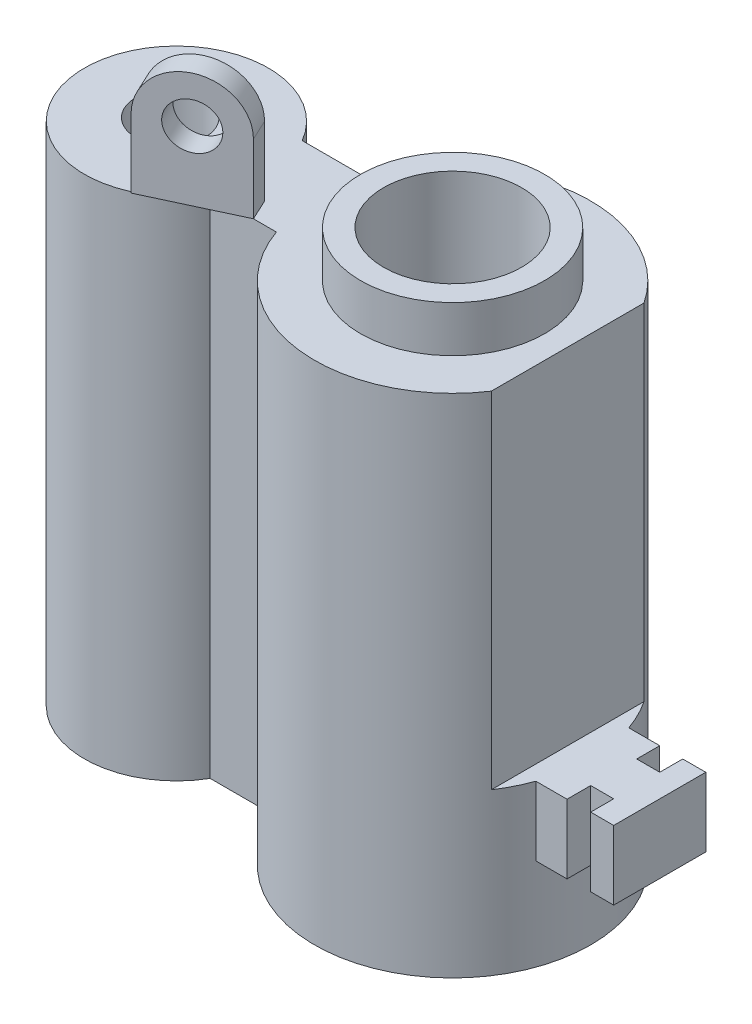
ISO-10303-21;
HEADER;
FILE_DESCRIPTION(('STEP AP214'),'2;1');
FILE_NAME('part.step','',(''),(''),'','','');
FILE_SCHEMA(('AUTOMOTIVE_DESIGN { 1 0 10303 214 1 1 1 1 }'));
ENDSEC;
DATA;
#1=APPLICATION_CONTEXT('core data for automotive mechanical design processes');
#2=APPLICATION_PROTOCOL_DEFINITION('international standard','automotive_design',2000,#1);
#3=PRODUCT_CONTEXT('',#1,'mechanical');
#4=PRODUCT('Part','Part','',(#3));
#5=PRODUCT_RELATED_PRODUCT_CATEGORY('part','',(#4));
#6=PRODUCT_DEFINITION_FORMATION('','',#4);
#7=PRODUCT_DEFINITION_CONTEXT('part definition',#1,'design');
#8=PRODUCT_DEFINITION('design','',#6,#7);
#9=PRODUCT_DEFINITION_SHAPE('','',#8);
#10=(LENGTH_UNIT() NAMED_UNIT(*) SI_UNIT(.MILLI.,.METRE.));
#11=(NAMED_UNIT(*) PLANE_ANGLE_UNIT() SI_UNIT($,.RADIAN.));
#12=(NAMED_UNIT(*) SI_UNIT($,.STERADIAN.) SOLID_ANGLE_UNIT());
#13=UNCERTAINTY_MEASURE_WITH_UNIT(LENGTH_MEASURE(1.E-05),#10,'distance_accuracy_value','');
#14=(GEOMETRIC_REPRESENTATION_CONTEXT(3) GLOBAL_UNCERTAINTY_ASSIGNED_CONTEXT((#13)) GLOBAL_UNIT_ASSIGNED_CONTEXT((#10,
#11,#12)) REPRESENTATION_CONTEXT('',''));
#15=CARTESIAN_POINT('',(0.,0.,0.));
#16=DIRECTION('',(0.,0.,1.));
#17=DIRECTION('',(1.,0.,0.));
#18=AXIS2_PLACEMENT_3D('',#15,#16,#17);
#19=CARTESIAN_POINT('',(0.,22.,0.));
#20=DIRECTION('',(0.,-1.,0.));
#21=DIRECTION('',(0.,0.,-1.));
#22=AXIS2_PLACEMENT_3D('',#19,#20,#21);
#23=CYLINDRICAL_SURFACE('',#22,6.);
#24=DIRECTION('',(0.,-1.,0.));
#25=VECTOR('',#24,1.);
#26=CARTESIAN_POINT('',(5.,27.,-3.3166247903554));
#27=LINE('',#26,#25);
#28=CARTESIAN_POINT('',(5.,22.,-3.3166247903554));
#29=VERTEX_POINT('',#28);
#30=CARTESIAN_POINT('',(5.,7.,-3.3166247903554));
#31=VERTEX_POINT('',#30);
#32=EDGE_CURVE('E215',#29,#31,#27,.T.);
#33=ORIENTED_EDGE('',*,*,#32,.T.);
#34=CARTESIAN_POINT('',(0.,7.,0.));
#35=DIRECTION('',(0.,1.,0.));
#36=DIRECTION('',(0.,0.,1.));
#37=AXIS2_PLACEMENT_3D('',#34,#35,#36);
#38=CIRCLE('',#37,6.);
#39=CARTESIAN_POINT('',(5.65685424949238,7.,-2.));
#40=VERTEX_POINT('',#39);
#41=EDGE_CURVE('E199',#40,#31,#38,.T.);
#42=ORIENTED_EDGE('',*,*,#41,.F.);
#43=DIRECTION('',(0.,1.,0.));
#44=VECTOR('',#43,1.);
#45=CARTESIAN_POINT('',(5.65685424949238,4.,-2.));
#46=LINE('',#45,#44);
#47=CARTESIAN_POINT('',(5.65685424949238,4.,-2.));
#48=VERTEX_POINT('',#47);
#49=EDGE_CURVE('E288',#48,#40,#46,.T.);
#50=ORIENTED_EDGE('',*,*,#49,.F.);
#51=CARTESIAN_POINT('',(0.,4.,0.));
#52=DIRECTION('',(0.,1.,0.));
#53=DIRECTION('',(0.,0.,1.));
#54=AXIS2_PLACEMENT_3D('',#51,#52,#53);
#55=CIRCLE('',#54,6.);
#56=CARTESIAN_POINT('',(5.64698166944062,4.,2.02770757877006));
#57=VERTEX_POINT('',#56);
#58=EDGE_CURVE('E46',#57,#48,#55,.T.);
#59=ORIENTED_EDGE('',*,*,#58,.F.);
#60=DIRECTION('',(0.,1.,0.));
#61=VECTOR('',#60,1.);
#62=CARTESIAN_POINT('',(5.64698166944062,4.,2.02770757877006));
#63=LINE('',#62,#61);
#64=CARTESIAN_POINT('',(5.64698166944062,7.,2.02770757877006));
#65=VERTEX_POINT('',#64);
#66=EDGE_CURVE('E259',#57,#65,#63,.T.);
#67=ORIENTED_EDGE('',*,*,#66,.T.);
#68=CARTESIAN_POINT('',(5.,7.,3.31662479035539));
#69=VERTEX_POINT('',#68);
#70=EDGE_CURVE('E206',#69,#65,#38,.T.);
#71=ORIENTED_EDGE('',*,*,#70,.F.);
#72=DIRECTION('',(0.,-1.,0.));
#73=VECTOR('',#72,1.);
#74=CARTESIAN_POINT('',(5.,27.,3.31662479035539));
#75=LINE('',#74,#73);
#76=CARTESIAN_POINT('',(5.,22.,3.31662479035539));
#77=VERTEX_POINT('',#76);
#78=EDGE_CURVE('E211',#77,#69,#75,.T.);
#79=ORIENTED_EDGE('',*,*,#78,.F.);
#80=CARTESIAN_POINT('',(0.,22.,0.));
#81=DIRECTION('',(0.,1.,0.));
#82=DIRECTION('',(0.,0.,1.));
#83=AXIS2_PLACEMENT_3D('',#80,#81,#82);
#84=CIRCLE('',#83,6.);
#85=CARTESIAN_POINT('',(-5.65685424949238,22.,2.));
#86=VERTEX_POINT('',#85);
#87=EDGE_CURVE('E373',#86,#77,#84,.T.);
#88=ORIENTED_EDGE('',*,*,#87,.F.);
#89=DIRECTION('',(0.,-1.,0.));
#90=VECTOR('',#89,1.);
#91=CARTESIAN_POINT('',(-5.65685424949238,22.,2.));
#92=LINE('',#91,#90);
#93=CARTESIAN_POINT('',(-5.65685424949238,0.,2.));
#94=VERTEX_POINT('',#93);
#95=EDGE_CURVE('E383',#86,#94,#92,.T.);
#96=ORIENTED_EDGE('',*,*,#95,.T.);
#97=CARTESIAN_POINT('',(0.,0.,0.));
#98=DIRECTION('',(0.,1.,0.));
#99=DIRECTION('',(0.,0.,1.));
#100=AXIS2_PLACEMENT_3D('',#97,#98,#99);
#101=CIRCLE('',#100,6.);
#102=CARTESIAN_POINT('',(-5.65685424949238,0.,-2.));
#103=VERTEX_POINT('',#102);
#104=EDGE_CURVE('E375',#94,#103,#101,.T.);
#105=ORIENTED_EDGE('',*,*,#104,.T.);
#106=DIRECTION('',(0.,-1.,0.));
#107=VECTOR('',#106,1.);
#108=CARTESIAN_POINT('',(-5.65685424949238,22.,-2.));
#109=LINE('',#108,#107);
#110=CARTESIAN_POINT('',(-5.65685424949238,22.,-2.));
#111=VERTEX_POINT('',#110);
#112=EDGE_CURVE('E405',#111,#103,#109,.T.);
#113=ORIENTED_EDGE('',*,*,#112,.F.);
#114=EDGE_CURVE('E220',#29,#111,#84,.T.);
#115=ORIENTED_EDGE('',*,*,#114,.F.);
#116=EDGE_LOOP('',(#33,#42,#50,#59,#67,#71,#79,#88,#96,#105,#113,#115));
#117=FACE_BOUND('',#116,.T.);
#118=ADVANCED_FACE('F39',(#117),#23,.T.);
#119=CARTESIAN_POINT('',(0.,22.,0.));
#120=DIRECTION('',(0.,1.,0.));
#121=DIRECTION('',(0.,0.,1.));
#122=AXIS2_PLACEMENT_3D('',#119,#120,#121);
#123=PLANE('',#122);
#124=CARTESIAN_POINT('',(0.,22.,0.));
#125=DIRECTION('',(0.,1.,0.));
#126=DIRECTION('',(0.,0.,1.));
#127=AXIS2_PLACEMENT_3D('',#124,#125,#126);
#128=CIRCLE('',#127,4.);
#129=CARTESIAN_POINT('',(0.,22.,4.));
#130=VERTEX_POINT('',#129);
#131=EDGE_CURVE('E317',#130,#130,#128,.T.);
#132=ORIENTED_EDGE('',*,*,#131,.F.);
#133=EDGE_LOOP('',(#132));
#134=FACE_BOUND('',#133,.T.);
#135=CARTESIAN_POINT('',(-12.2679491924311,22.,0.));
#136=DIRECTION('',(0.,1.,0.));
#137=DIRECTION('',(0.,0.,1.));
#138=AXIS2_PLACEMENT_3D('',#135,#136,#137);
#139=CIRCLE('',#138,1.5);
#140=CARTESIAN_POINT('',(-12.2679491924311,22.,1.5));
#141=VERTEX_POINT('',#140);
#142=EDGE_CURVE('E333',#141,#141,#139,.T.);
#143=ORIENTED_EDGE('',*,*,#142,.F.);
#144=EDGE_LOOP('',(#143));
#145=FACE_BOUND('',#144,.T.);
#146=ORIENTED_EDGE('',*,*,#87,.T.);
#147=DIRECTION('',(0.,0.,-1.));
#148=VECTOR('',#147,1.);
#149=CARTESIAN_POINT('',(5.,22.,0.));
#150=LINE('',#149,#148);
#151=EDGE_CURVE('E11',#77,#29,#150,.T.);
#152=ORIENTED_EDGE('',*,*,#151,.T.);
#153=ORIENTED_EDGE('',*,*,#114,.T.);
#154=DIRECTION('',(-1.,0.,0.));
#155=VECTOR('',#154,1.);
#156=CARTESIAN_POINT('',(-8.53589838486226,22.,-2.));
#157=LINE('',#156,#155);
#158=CARTESIAN_POINT('',(-8.53589838486226,22.,-2.));
#159=VERTEX_POINT('',#158);
#160=EDGE_CURVE('E376',#111,#159,#157,.T.);
#161=ORIENTED_EDGE('',*,*,#160,.T.);
#162=CARTESIAN_POINT('',(-12.,22.,0.));
#163=DIRECTION('',(0.,1.,0.));
#164=DIRECTION('',(0.,0.,1.));
#165=AXIS2_PLACEMENT_3D('',#162,#163,#164);
#166=CIRCLE('',#165,3.99999999999999);
#167=CARTESIAN_POINT('',(-10.3095269530372,22.,3.6252311481466));
#168=VERTEX_POINT('',#167);
#169=EDGE_CURVE('E378',#159,#168,#166,.T.);
#170=ORIENTED_EDGE('',*,*,#169,.T.);
#171=DIRECTION('',(0.422618261740698,0.,0.906307787036651));
#172=VECTOR('',#171,1.);
#173=CARTESIAN_POINT('',(-10.2791041559867,22.,3.69047304696279));
#174=LINE('',#173,#172);
#175=CARTESIAN_POINT('',(-10.7017224177274,22.,2.78416525992614));
#176=VERTEX_POINT('',#175);
#177=EDGE_CURVE('E52',#176,#168,#174,.T.);
#178=ORIENTED_EDGE('',*,*,#177,.F.);
#179=DIRECTION('',(-0.906307787036651,0.,0.422618261740697));
#180=VECTOR('',#179,1.);
#181=CARTESIAN_POINT('',(-10.7017224177274,22.,2.78416525992614));
#182=LINE('',#181,#180);
#183=CARTESIAN_POINT('',(-7.07649126958075,22.,1.09369221296335));
#184=VERTEX_POINT('',#183);
#185=EDGE_CURVE('E353',#184,#176,#182,.T.);
#186=ORIENTED_EDGE('',*,*,#185,.F.);
#187=DIRECTION('',(-0.422618261740697,0.,-0.906307787036651));
#188=VECTOR('',#187,1.);
#189=CARTESIAN_POINT('',(-7.07649126958075,22.,1.09369221296335));
#190=LINE('',#189,#188);
#191=CARTESIAN_POINT('',(-6.65387300784006,22.,2.));
#192=VERTEX_POINT('',#191);
#193=EDGE_CURVE('E56',#192,#184,#190,.T.);
#194=ORIENTED_EDGE('',*,*,#193,.F.);
#195=DIRECTION('',(1.,0.,0.));
#196=VECTOR('',#195,1.);
#197=CARTESIAN_POINT('',(-8.53589838486226,22.,2.));
#198=LINE('',#197,#196);
#199=EDGE_CURVE('E382',#192,#86,#198,.T.);
#200=ORIENTED_EDGE('',*,*,#199,.T.);
#201=EDGE_LOOP('',(#146,#152,#153,#161,#170,#178,#186,#194,#200));
#202=FACE_BOUND('',#201,.T.);
#203=ADVANCED_FACE('F452',(#134,#145,#202),#123,.T.);
#204=CARTESIAN_POINT('',(-8.53589838486226,22.,-2.));
#205=DIRECTION('',(0.,0.,1.));
#206=DIRECTION('',(1.,0.,0.));
#207=AXIS2_PLACEMENT_3D('',#204,#205,#206);
#208=PLANE('',#207);
#209=DIRECTION('',(-1.,0.,0.));
#210=VECTOR('',#209,1.);
#211=CARTESIAN_POINT('',(-8.53589838486226,0.,-2.));
#212=LINE('',#211,#210);
#213=CARTESIAN_POINT('',(-8.53589838486226,0.,-2.));
#214=VERTEX_POINT('',#213);
#215=EDGE_CURVE('E389',#103,#214,#212,.T.);
#216=ORIENTED_EDGE('',*,*,#215,.T.);
#217=DIRECTION('',(0.,-1.,0.));
#218=VECTOR('',#217,1.);
#219=CARTESIAN_POINT('',(-8.53589838486226,22.,-2.));
#220=LINE('',#219,#218);
#221=EDGE_CURVE('E399',#159,#214,#220,.T.);
#222=ORIENTED_EDGE('',*,*,#221,.F.);
#223=ORIENTED_EDGE('',*,*,#160,.F.);
#224=ORIENTED_EDGE('',*,*,#112,.T.);
#225=EDGE_LOOP('',(#216,#222,#223,#224));
#226=FACE_BOUND('',#225,.T.);
#227=ADVANCED_FACE('F464',(#226),#208,.F.);
#228=CARTESIAN_POINT('',(-12.,22.,0.));
#229=DIRECTION('',(0.,-1.,0.));
#230=DIRECTION('',(0.,0.,-1.));
#231=AXIS2_PLACEMENT_3D('',#228,#229,#230);
#232=CYLINDRICAL_SURFACE('',#231,3.99999999999999);
#233=CARTESIAN_POINT('',(-12.,0.,0.));
#234=DIRECTION('',(0.,1.,0.));
#235=DIRECTION('',(0.,0.,1.));
#236=AXIS2_PLACEMENT_3D('',#233,#234,#235);
#237=CIRCLE('',#236,3.99999999999999);
#238=CARTESIAN_POINT('',(-8.53589838486226,0.,2.));
#239=VERTEX_POINT('',#238);
#240=EDGE_CURVE('E388',#214,#239,#237,.T.);
#241=ORIENTED_EDGE('',*,*,#240,.T.);
#242=DIRECTION('',(0.,-1.,0.));
#243=VECTOR('',#242,1.);
#244=CARTESIAN_POINT('',(-8.53589838486226,22.,2.));
#245=LINE('',#244,#243);
#246=CARTESIAN_POINT('',(-8.53589838486226,22.,2.));
#247=VERTEX_POINT('',#246);
#248=EDGE_CURVE('E398',#247,#239,#245,.T.);
#249=ORIENTED_EDGE('',*,*,#248,.F.);
#250=EDGE_CURVE('E377',#168,#247,#166,.T.);
#251=ORIENTED_EDGE('',*,*,#250,.F.);
#252=ORIENTED_EDGE('',*,*,#169,.F.);
#253=ORIENTED_EDGE('',*,*,#221,.T.);
#254=EDGE_LOOP('',(#241,#249,#251,#252,#253));
#255=FACE_BOUND('',#254,.T.);
#256=ADVANCED_FACE('F509',(#255),#232,.T.);
#257=CARTESIAN_POINT('',(-8.53589838486226,22.,2.));
#258=DIRECTION('',(0.,0.,-1.));
#259=DIRECTION('',(-1.,0.,0.));
#260=AXIS2_PLACEMENT_3D('',#257,#258,#259);
#261=PLANE('',#260);
#262=DIRECTION('',(1.,0.,0.));
#263=VECTOR('',#262,1.);
#264=CARTESIAN_POINT('',(-8.53589838486226,0.,2.));
#265=LINE('',#264,#263);
#266=EDGE_CURVE('E391',#239,#94,#265,.T.);
#267=ORIENTED_EDGE('',*,*,#266,.T.);
#268=ORIENTED_EDGE('',*,*,#95,.F.);
#269=ORIENTED_EDGE('',*,*,#199,.F.);
#270=EDGE_CURVE('E385',#247,#192,#198,.T.);
#271=ORIENTED_EDGE('',*,*,#270,.F.);
#272=ORIENTED_EDGE('',*,*,#248,.T.);
#273=EDGE_LOOP('',(#267,#268,#269,#271,#272));
#274=FACE_BOUND('',#273,.T.);
#275=ADVANCED_FACE('F453',(#274),#261,.F.);
#276=CARTESIAN_POINT('',(0.,0.,0.));
#277=DIRECTION('',(0.,1.,0.));
#278=DIRECTION('',(0.,0.,1.));
#279=AXIS2_PLACEMENT_3D('',#276,#277,#278);
#280=PLANE('',#279);
#281=CARTESIAN_POINT('',(0.,0.,0.));
#282=DIRECTION('',(0.,1.,0.));
#283=DIRECTION('',(0.,0.,1.));
#284=AXIS2_PLACEMENT_3D('',#281,#282,#283);
#285=CIRCLE('',#284,3.);
#286=CARTESIAN_POINT('',(0.,0.,3.));
#287=VERTEX_POINT('',#286);
#288=EDGE_CURVE('E286',#287,#287,#285,.T.);
#289=ORIENTED_EDGE('',*,*,#288,.T.);
#290=EDGE_LOOP('',(#289));
#291=FACE_BOUND('',#290,.T.);
#292=CARTESIAN_POINT('',(-12.2679491924311,0.,0.));
#293=DIRECTION('',(0.,1.,0.));
#294=DIRECTION('',(0.,0.,1.));
#295=AXIS2_PLACEMENT_3D('',#292,#293,#294);
#296=CIRCLE('',#295,1.5);
#297=CARTESIAN_POINT('',(-12.2679491924311,0.,1.5));
#298=VERTEX_POINT('',#297);
#299=EDGE_CURVE('E323',#298,#298,#296,.T.);
#300=ORIENTED_EDGE('',*,*,#299,.T.);
#301=EDGE_LOOP('',(#300));
#302=FACE_BOUND('',#301,.T.);
#303=ORIENTED_EDGE('',*,*,#104,.F.);
#304=ORIENTED_EDGE('',*,*,#266,.F.);
#305=ORIENTED_EDGE('',*,*,#240,.F.);
#306=ORIENTED_EDGE('',*,*,#215,.F.);
#307=EDGE_LOOP('',(#303,#304,#305,#306));
#308=FACE_BOUND('',#307,.T.);
#309=ADVANCED_FACE('F458',(#291,#302,#308),#280,.F.);
#310=CARTESIAN_POINT('',(-10.2791041559867,25.,3.69047304696279));
#311=DIRECTION('',(0.906307787036651,0.,-0.422618261740698));
#312=DIRECTION('',(-0.422618261740698,0.,-0.906307787036651));
#313=AXIS2_PLACEMENT_3D('',#310,#311,#312);
#314=PLANE('',#313);
#315=ORIENTED_EDGE('',*,*,#177,.T.);
#316=CARTESIAN_POINT('',(-10.2791041559867,22.,3.69047304696279));
#317=VERTEX_POINT('',#316);
#318=EDGE_CURVE('E341',#168,#317,#174,.T.);
#319=ORIENTED_EDGE('',*,*,#318,.T.);
#320=DIRECTION('',(0.,-1.,0.));
#321=VECTOR('',#320,1.);
#322=CARTESIAN_POINT('',(-10.2791041559867,25.,3.69047304696279));
#323=LINE('',#322,#321);
#324=CARTESIAN_POINT('',(-10.2791041559867,25.,3.69047304696279));
#325=VERTEX_POINT('',#324);
#326=EDGE_CURVE('E367',#325,#317,#323,.T.);
#327=ORIENTED_EDGE('',*,*,#326,.F.);
#328=DIRECTION('',(0.422618261740698,0.,0.906307787036651));
#329=VECTOR('',#328,1.);
#330=CARTESIAN_POINT('',(-10.2791041559867,25.,3.69047304696279));
#331=LINE('',#330,#329);
#332=CARTESIAN_POINT('',(-10.7017224177274,25.,2.78416525992614));
#333=VERTEX_POINT('',#332);
#334=EDGE_CURVE('E346',#333,#325,#331,.T.);
#335=ORIENTED_EDGE('',*,*,#334,.F.);
#336=DIRECTION('',(0.,-1.,0.));
#337=VECTOR('',#336,1.);
#338=CARTESIAN_POINT('',(-10.7017224177274,25.,2.78416525992614));
#339=LINE('',#338,#337);
#340=EDGE_CURVE('E354',#333,#176,#339,.T.);
#341=ORIENTED_EDGE('',*,*,#340,.T.);
#342=EDGE_LOOP('',(#315,#319,#327,#335,#341));
#343=FACE_BOUND('',#342,.T.);
#344=ADVANCED_FACE('F474',(#343),#314,.F.);
#345=CARTESIAN_POINT('',(-6.65387300784006,25.,2.));
#346=DIRECTION('',(-0.422618261740697,0.,-0.906307787036651));
#347=DIRECTION('',(-0.906307787036651,0.,0.422618261740698));
#348=AXIS2_PLACEMENT_3D('',#345,#346,#347);
#349=PLANE('',#348);
#350=CARTESIAN_POINT('',(-8.46648858191335,25.,2.8452365234814));
#351=DIRECTION('',(0.422618261740698,0.,0.906307787036651));
#352=DIRECTION('',(0.906307787036651,0.,-0.422618261740698));
#353=AXIS2_PLACEMENT_3D('',#350,#351,#352);
#354=CIRCLE('',#353,1.);
#355=CARTESIAN_POINT('',(-7.5601807948767,25.,2.4226182617407));
#356=VERTEX_POINT('',#355);
#357=EDGE_CURVE('E334',#356,#356,#354,.T.);
#358=ORIENTED_EDGE('',*,*,#357,.F.);
#359=EDGE_LOOP('',(#358));
#360=FACE_BOUND('',#359,.T.);
#361=DIRECTION('',(0.906307787036651,0.,-0.422618261740697));
#362=VECTOR('',#361,1.);
#363=CARTESIAN_POINT('',(-6.65387300784006,22.,2.));
#364=LINE('',#363,#362);
#365=EDGE_CURVE('E358',#317,#192,#364,.T.);
#366=ORIENTED_EDGE('',*,*,#365,.T.);
#367=DIRECTION('',(0.,-1.,0.));
#368=VECTOR('',#367,1.);
#369=CARTESIAN_POINT('',(-6.65387300784006,25.,2.));
#370=LINE('',#369,#368);
#371=CARTESIAN_POINT('',(-6.65387300784006,25.,2.));
#372=VERTEX_POINT('',#371);
#373=EDGE_CURVE('E366',#372,#192,#370,.T.);
#374=ORIENTED_EDGE('',*,*,#373,.F.);
#375=CARTESIAN_POINT('',(-8.46648858191336,25.,2.8452365234814));
#376=DIRECTION('',(0.422618261740698,0.,0.906307787036651));
#377=DIRECTION('',(0.906307787036651,0.,-0.422618261740698));
#378=AXIS2_PLACEMENT_3D('',#375,#376,#377);
#379=CIRCLE('',#378,2.);
#380=EDGE_CURVE('E336',#372,#325,#379,.T.);
#381=ORIENTED_EDGE('',*,*,#380,.T.);
#382=ORIENTED_EDGE('',*,*,#326,.T.);
#383=EDGE_LOOP('',(#366,#374,#381,#382));
#384=FACE_BOUND('',#383,.T.);
#385=ADVANCED_FACE('F481',(#360,#384),#349,.F.);
#386=CARTESIAN_POINT('',(-7.07649126958075,25.,1.09369221296335));
#387=DIRECTION('',(-0.906307787036651,0.,0.422618261740697));
#388=DIRECTION('',(0.422618261740697,0.,0.906307787036651));
#389=AXIS2_PLACEMENT_3D('',#386,#387,#388);
#390=PLANE('',#389);
#391=ORIENTED_EDGE('',*,*,#193,.T.);
#392=DIRECTION('',(0.,-1.,0.));
#393=VECTOR('',#392,1.);
#394=CARTESIAN_POINT('',(-7.07649126958075,25.,1.09369221296335));
#395=LINE('',#394,#393);
#396=CARTESIAN_POINT('',(-7.07649126958075,25.,1.09369221296335));
#397=VERTEX_POINT('',#396);
#398=EDGE_CURVE('E361',#397,#184,#395,.T.);
#399=ORIENTED_EDGE('',*,*,#398,.F.);
#400=DIRECTION('',(-0.422618261740697,0.,-0.906307787036651));
#401=VECTOR('',#400,1.);
#402=CARTESIAN_POINT('',(-7.07649126958075,25.,1.09369221296335));
#403=LINE('',#402,#401);
#404=EDGE_CURVE('E347',#372,#397,#403,.T.);
#405=ORIENTED_EDGE('',*,*,#404,.F.);
#406=ORIENTED_EDGE('',*,*,#373,.T.);
#407=EDGE_LOOP('',(#391,#399,#405,#406));
#408=FACE_BOUND('',#407,.T.);
#409=ADVANCED_FACE('F478',(#408),#390,.F.);
#410=CARTESIAN_POINT('',(-10.7017224177274,25.,2.78416525992614));
#411=DIRECTION('',(0.422618261740697,0.,0.906307787036651));
#412=DIRECTION('',(0.906307787036651,0.,-0.422618261740697));
#413=AXIS2_PLACEMENT_3D('',#410,#411,#412);
#414=PLANE('',#413);
#415=CARTESIAN_POINT('',(-8.88910684365405,25.,1.93892873644474));
#416=DIRECTION('',(0.422618261740698,0.,0.906307787036651));
#417=DIRECTION('',(0.906307787036651,0.,-0.422618261740698));
#418=AXIS2_PLACEMENT_3D('',#415,#416,#417);
#419=CIRCLE('',#418,1.);
#420=CARTESIAN_POINT('',(-7.9827990566174,25.,1.51631047470405));
#421=VERTEX_POINT('',#420);
#422=EDGE_CURVE('E332',#421,#421,#419,.T.);
#423=ORIENTED_EDGE('',*,*,#422,.T.);
#424=EDGE_LOOP('',(#423));
#425=FACE_BOUND('',#424,.T.);
#426=ORIENTED_EDGE('',*,*,#185,.T.);
#427=ORIENTED_EDGE('',*,*,#340,.F.);
#428=CARTESIAN_POINT('',(-8.88910684365406,25.,1.93892873644475));
#429=DIRECTION('',(0.422618261740698,0.,0.906307787036651));
#430=DIRECTION('',(0.906307787036651,0.,-0.422618261740698));
#431=AXIS2_PLACEMENT_3D('',#428,#429,#430);
#432=CIRCLE('',#431,2.);
#433=EDGE_CURVE('E342',#397,#333,#432,.T.);
#434=ORIENTED_EDGE('',*,*,#433,.F.);
#435=ORIENTED_EDGE('',*,*,#398,.T.);
#436=EDGE_LOOP('',(#426,#427,#434,#435));
#437=FACE_BOUND('',#436,.T.);
#438=ADVANCED_FACE('F476',(#425,#437),#414,.F.);
#439=CARTESIAN_POINT('',(0.,22.,0.));
#440=DIRECTION('',(0.,-1.,0.));
#441=DIRECTION('',(0.,0.,-1.));
#442=AXIS2_PLACEMENT_3D('',#439,#440,#441);
#443=PLANE('',#442);
#444=ORIENTED_EDGE('',*,*,#318,.F.);
#445=ORIENTED_EDGE('',*,*,#250,.T.);
#446=ORIENTED_EDGE('',*,*,#270,.T.);
#447=ORIENTED_EDGE('',*,*,#365,.F.);
#448=EDGE_LOOP('',(#444,#445,#446,#447));
#449=FACE_BOUND('',#448,.T.);
#450=ADVANCED_FACE('F472',(#449),#443,.T.);
#451=CARTESIAN_POINT('',(-8.88910684365406,25.,1.93892873644475));
#452=DIRECTION('',(0.422618261740698,0.,0.906307787036651));
#453=DIRECTION('',(0.906307787036651,0.,-0.422618261740698));
#454=AXIS2_PLACEMENT_3D('',#451,#452,#453);
#455=CYLINDRICAL_SURFACE('',#454,2.);
#456=ORIENTED_EDGE('',*,*,#380,.F.);
#457=ORIENTED_EDGE('',*,*,#404,.T.);
#458=ORIENTED_EDGE('',*,*,#433,.T.);
#459=ORIENTED_EDGE('',*,*,#334,.T.);
#460=EDGE_LOOP('',(#456,#457,#458,#459));
#461=FACE_BOUND('',#460,.T.);
#462=ADVANCED_FACE('F482',(#461),#455,.T.);
#463=CARTESIAN_POINT('',(-8.88910684365405,25.,1.93892873644474));
#464=DIRECTION('',(0.422618261740698,0.,0.906307787036651));
#465=DIRECTION('',(0.906307787036651,0.,-0.422618261740698));
#466=AXIS2_PLACEMENT_3D('',#463,#464,#465);
#467=CYLINDRICAL_SURFACE('',#466,1.);
#468=ORIENTED_EDGE('',*,*,#422,.F.);
#469=EDGE_LOOP('',(#468));
#470=FACE_BOUND('',#469,.T.);
#471=ORIENTED_EDGE('',*,*,#357,.T.);
#472=EDGE_LOOP('',(#471));
#473=FACE_BOUND('',#472,.T.);
#474=ADVANCED_FACE('F487',(#470,#473),#467,.F.);
#475=CARTESIAN_POINT('',(-12.2679491924311,22.,0.));
#476=DIRECTION('',(0.,1.,0.));
#477=DIRECTION('',(0.,0.,1.));
#478=AXIS2_PLACEMENT_3D('',#475,#476,#477);
#479=CYLINDRICAL_SURFACE('',#478,1.5);
#480=CARTESIAN_POINT('',(-12.2679491924311,16.,0.));
#481=DIRECTION('',(0.,1.,0.));
#482=DIRECTION('',(0.,0.,1.));
#483=AXIS2_PLACEMENT_3D('',#480,#481,#482);
#484=CIRCLE('',#483,1.5);
#485=CARTESIAN_POINT('',(-12.2679491924311,16.,1.5));
#486=VERTEX_POINT('',#485);
#487=EDGE_CURVE('E330',#486,#486,#484,.T.);
#488=ORIENTED_EDGE('',*,*,#487,.F.);
#489=EDGE_LOOP('',(#488));
#490=FACE_BOUND('',#489,.T.);
#491=ORIENTED_EDGE('',*,*,#142,.T.);
#492=EDGE_LOOP('',(#491));
#493=FACE_BOUND('',#492,.T.);
#494=ADVANCED_FACE('F494',(#490,#493),#479,.F.);
#495=CARTESIAN_POINT('',(-12.2679491924311,16.,0.));
#496=DIRECTION('',(0.,1.,0.));
#497=DIRECTION('',(0.,0.,1.));
#498=AXIS2_PLACEMENT_3D('',#495,#496,#497);
#499=CONICAL_SURFACE('',#498,1.5,0.982793723247328);
#500=CARTESIAN_POINT('',(-12.2679491924311,15.,0.));
#501=VERTEX_POINT('',#500);
#502=VERTEX_LOOP('',#501);
#503=FACE_BOUND('',#502,.T.);
#504=ORIENTED_EDGE('',*,*,#487,.T.);
#505=EDGE_LOOP('',(#504));
#506=FACE_BOUND('',#505,.T.);
#507=ADVANCED_FACE('F593',(#503,#506),#499,.F.);
#508=CARTESIAN_POINT('',(-12.2679491924311,0.,0.));
#509=DIRECTION('',(0.,-1.,0.));
#510=DIRECTION('',(0.,0.,1.));
#511=AXIS2_PLACEMENT_3D('',#508,#509,#510);
#512=CYLINDRICAL_SURFACE('',#511,1.5);
#513=CARTESIAN_POINT('',(-12.2679491924311,6.,0.));
#514=DIRECTION('',(0.,1.,0.));
#515=DIRECTION('',(0.,0.,1.));
#516=AXIS2_PLACEMENT_3D('',#513,#514,#515);
#517=CIRCLE('',#516,1.5);
#518=CARTESIAN_POINT('',(-12.2679491924311,6.,1.5));
#519=VERTEX_POINT('',#518);
#520=EDGE_CURVE('E318',#519,#519,#517,.T.);
#521=ORIENTED_EDGE('',*,*,#520,.T.);
#522=EDGE_LOOP('',(#521));
#523=FACE_BOUND('',#522,.T.);
#524=ORIENTED_EDGE('',*,*,#299,.F.);
#525=EDGE_LOOP('',(#524));
#526=FACE_BOUND('',#525,.T.);
#527=ADVANCED_FACE('F602',(#523,#526),#512,.F.);
#528=CARTESIAN_POINT('',(-12.2679491924311,6.,0.));
#529=DIRECTION('',(0.,-1.,0.));
#530=DIRECTION('',(0.,0.,1.));
#531=AXIS2_PLACEMENT_3D('',#528,#529,#530);
#532=CONICAL_SURFACE('',#531,1.5,0.982793723247328);
#533=CARTESIAN_POINT('',(-12.2679491924311,7.,0.));
#534=VERTEX_POINT('',#533);
#535=VERTEX_LOOP('',#534);
#536=FACE_BOUND('',#535,.T.);
#537=ORIENTED_EDGE('',*,*,#520,.F.);
#538=EDGE_LOOP('',(#537));
#539=FACE_BOUND('',#538,.T.);
#540=ADVANCED_FACE('F613',(#536,#539),#532,.F.);
#541=CARTESIAN_POINT('',(0.,24.,0.));
#542=DIRECTION('',(0.,1.,0.));
#543=DIRECTION('',(0.,0.,1.));
#544=AXIS2_PLACEMENT_3D('',#541,#542,#543);
#545=PLANE('',#544);
#546=CARTESIAN_POINT('',(0.,24.,0.));
#547=DIRECTION('',(0.,1.,0.));
#548=DIRECTION('',(0.,0.,1.));
#549=AXIS2_PLACEMENT_3D('',#546,#547,#548);
#550=CIRCLE('',#549,4.);
#551=CARTESIAN_POINT('',(0.,24.,4.));
#552=VERTEX_POINT('',#551);
#553=EDGE_CURVE('E320',#552,#552,#550,.T.);
#554=ORIENTED_EDGE('',*,*,#553,.T.);
#555=EDGE_LOOP('',(#554));
#556=FACE_BOUND('',#555,.T.);
#557=CARTESIAN_POINT('',(0.,24.,0.));
#558=DIRECTION('',(0.,1.,0.));
#559=DIRECTION('',(0.,0.,1.));
#560=AXIS2_PLACEMENT_3D('',#557,#558,#559);
#561=CIRCLE('',#560,3.);
#562=CARTESIAN_POINT('',(0.,24.,3.));
#563=VERTEX_POINT('',#562);
#564=EDGE_CURVE('E312',#563,#563,#561,.T.);
#565=ORIENTED_EDGE('',*,*,#564,.F.);
#566=EDGE_LOOP('',(#565));
#567=FACE_BOUND('',#566,.T.);
#568=ADVANCED_FACE('F623',(#556,#567),#545,.T.);
#569=CARTESIAN_POINT('',(0.,24.,0.));
#570=DIRECTION('',(0.,-1.,0.));
#571=DIRECTION('',(0.,0.,-1.));
#572=AXIS2_PLACEMENT_3D('',#569,#570,#571);
#573=CYLINDRICAL_SURFACE('',#572,4.);
#574=ORIENTED_EDGE('',*,*,#553,.F.);
#575=EDGE_LOOP('',(#574));
#576=FACE_BOUND('',#575,.T.);
#577=ORIENTED_EDGE('',*,*,#131,.T.);
#578=EDGE_LOOP('',(#577));
#579=FACE_BOUND('',#578,.T.);
#580=ADVANCED_FACE('F631',(#576,#579),#573,.T.);
#581=CARTESIAN_POINT('',(0.,24.,0.));
#582=DIRECTION('',(0.,-1.,0.));
#583=DIRECTION('',(0.,0.,-1.));
#584=AXIS2_PLACEMENT_3D('',#581,#582,#583);
#585=CYLINDRICAL_SURFACE('',#584,3.);
#586=ORIENTED_EDGE('',*,*,#564,.T.);
#587=EDGE_LOOP('',(#586));
#588=FACE_BOUND('',#587,.T.);
#589=ORIENTED_EDGE('',*,*,#288,.F.);
#590=EDGE_LOOP('',(#589));
#591=FACE_BOUND('',#590,.T.);
#592=ADVANCED_FACE('F642',(#588,#591),#585,.F.);
#593=CARTESIAN_POINT('',(0.,4.,0.));
#594=DIRECTION('',(0.,1.,0.));
#595=DIRECTION('',(0.,0.,1.));
#596=AXIS2_PLACEMENT_3D('',#593,#594,#595);
#597=PLANE('',#596);
#598=DIRECTION('',(1.,0.,0.));
#599=VECTOR('',#598,1.);
#600=CARTESIAN_POINT('',(7.,4.,2.02770757877006));
#601=LINE('',#600,#599);
#602=CARTESIAN_POINT('',(7.,4.,2.02770757877006));
#603=VERTEX_POINT('',#602);
#604=EDGE_CURVE('E228',#57,#603,#601,.T.);
#605=ORIENTED_EDGE('',*,*,#604,.F.);
#606=ORIENTED_EDGE('',*,*,#58,.T.);
#607=DIRECTION('',(-1.,0.,0.));
#608=VECTOR('',#607,1.);
#609=CARTESIAN_POINT('',(7.,4.,-2.));
#610=LINE('',#609,#608);
#611=CARTESIAN_POINT('',(7.,4.,-2.));
#612=VERTEX_POINT('',#611);
#613=EDGE_CURVE('E257',#612,#48,#610,.T.);
#614=ORIENTED_EDGE('',*,*,#613,.F.);
#615=DIRECTION('',(0.,0.,-1.));
#616=VECTOR('',#615,1.);
#617=CARTESIAN_POINT('',(7.,4.,-1.));
#618=LINE('',#617,#616);
#619=CARTESIAN_POINT('',(7.,4.,-1.));
#620=VERTEX_POINT('',#619);
#621=EDGE_CURVE('E254',#620,#612,#618,.T.);
#622=ORIENTED_EDGE('',*,*,#621,.F.);
#623=DIRECTION('',(-1.,0.,0.));
#624=VECTOR('',#623,1.);
#625=CARTESIAN_POINT('',(8.,4.,-1.));
#626=LINE('',#625,#624);
#627=CARTESIAN_POINT('',(8.,4.,-1.));
#628=VERTEX_POINT('',#627);
#629=EDGE_CURVE('E249',#628,#620,#626,.T.);
#630=ORIENTED_EDGE('',*,*,#629,.F.);
#631=DIRECTION('',(0.,0.,1.));
#632=VECTOR('',#631,1.);
#633=CARTESIAN_POINT('',(8.,4.,-2.));
#634=LINE('',#633,#632);
#635=CARTESIAN_POINT('',(8.,4.,-2.));
#636=VERTEX_POINT('',#635);
#637=EDGE_CURVE('E250',#636,#628,#634,.T.);
#638=ORIENTED_EDGE('',*,*,#637,.F.);
#639=DIRECTION('',(-1.,0.,0.));
#640=VECTOR('',#639,1.);
#641=CARTESIAN_POINT('',(9.,4.,-2.));
#642=LINE('',#641,#640);
#643=CARTESIAN_POINT('',(9.,4.,-2.));
#644=VERTEX_POINT('',#643);
#645=EDGE_CURVE('E242',#644,#636,#642,.T.);
#646=ORIENTED_EDGE('',*,*,#645,.F.);
#647=DIRECTION('',(0.,0.,-1.));
#648=VECTOR('',#647,1.);
#649=CARTESIAN_POINT('',(9.,4.,-2.));
#650=LINE('',#649,#648);
#651=CARTESIAN_POINT('',(9.,4.,2.));
#652=VERTEX_POINT('',#651);
#653=EDGE_CURVE('E241',#652,#644,#650,.T.);
#654=ORIENTED_EDGE('',*,*,#653,.F.);
#655=DIRECTION('',(1.,0.,0.));
#656=VECTOR('',#655,1.);
#657=CARTESIAN_POINT('',(9.,4.,2.));
#658=LINE('',#657,#656);
#659=CARTESIAN_POINT('',(8.,4.,2.));
#660=VERTEX_POINT('',#659);
#661=EDGE_CURVE('E238',#660,#652,#658,.T.);
#662=ORIENTED_EDGE('',*,*,#661,.F.);
#663=DIRECTION('',(0.,0.,1.));
#664=VECTOR('',#663,1.);
#665=CARTESIAN_POINT('',(8.,4.,2.));
#666=LINE('',#665,#664);
#667=CARTESIAN_POINT('',(8.,4.,0.999999999999998));
#668=VERTEX_POINT('',#667);
#669=EDGE_CURVE('E232',#668,#660,#666,.T.);
#670=ORIENTED_EDGE('',*,*,#669,.F.);
#671=DIRECTION('',(1.,0.,0.));
#672=VECTOR('',#671,1.);
#673=CARTESIAN_POINT('',(8.,4.,0.999999999999998));
#674=LINE('',#673,#672);
#675=CARTESIAN_POINT('',(7.,4.,0.999999999999999));
#676=VERTEX_POINT('',#675);
#677=EDGE_CURVE('E235',#676,#668,#674,.T.);
#678=ORIENTED_EDGE('',*,*,#677,.F.);
#679=DIRECTION('',(0.,0.,-1.));
#680=VECTOR('',#679,1.);
#681=CARTESIAN_POINT('',(7.,4.,0.999999999999999));
#682=LINE('',#681,#680);
#683=EDGE_CURVE('E230',#603,#676,#682,.T.);
#684=ORIENTED_EDGE('',*,*,#683,.F.);
#685=EDGE_LOOP('',(#605,#606,#614,#622,#630,#638,#646,#654,#662,#670,#678,#684));
#686=FACE_BOUND('',#685,.T.);
#687=ADVANCED_FACE('F409',(#686),#597,.F.);
#688=CARTESIAN_POINT('',(0.,7.,0.));
#689=DIRECTION('',(0.,1.,0.));
#690=DIRECTION('',(0.,0.,1.));
#691=AXIS2_PLACEMENT_3D('',#688,#689,#690);
#692=PLANE('',#691);
#693=DIRECTION('',(-1.,0.,0.));
#694=VECTOR('',#693,1.);
#695=CARTESIAN_POINT('',(7.,7.,-2.));
#696=LINE('',#695,#694);
#697=CARTESIAN_POINT('',(7.,7.,-2.));
#698=VERTEX_POINT('',#697);
#699=EDGE_CURVE('E201',#698,#40,#696,.T.);
#700=ORIENTED_EDGE('',*,*,#699,.T.);
#701=ORIENTED_EDGE('',*,*,#41,.T.);
#702=DIRECTION('',(0.,0.,1.));
#703=VECTOR('',#702,1.);
#704=CARTESIAN_POINT('',(5.,7.,-3.3166247903554));
#705=LINE('',#704,#703);
#706=EDGE_CURVE('E198',#31,#69,#705,.T.);
#707=ORIENTED_EDGE('',*,*,#706,.T.);
#708=ORIENTED_EDGE('',*,*,#70,.T.);
#709=DIRECTION('',(1.,0.,0.));
#710=VECTOR('',#709,1.);
#711=CARTESIAN_POINT('',(7.,7.,2.02770757877006));
#712=LINE('',#711,#710);
#713=CARTESIAN_POINT('',(7.,7.,2.02770757877006));
#714=VERTEX_POINT('',#713);
#715=EDGE_CURVE('E218',#65,#714,#712,.T.);
#716=ORIENTED_EDGE('',*,*,#715,.T.);
#717=DIRECTION('',(0.,0.,-1.));
#718=VECTOR('',#717,1.);
#719=CARTESIAN_POINT('',(7.,7.,0.999999999999999));
#720=LINE('',#719,#718);
#721=CARTESIAN_POINT('',(7.,7.,0.999999999999999));
#722=VERTEX_POINT('',#721);
#723=EDGE_CURVE('E225',#714,#722,#720,.T.);
#724=ORIENTED_EDGE('',*,*,#723,.T.);
#725=DIRECTION('',(1.,0.,0.));
#726=VECTOR('',#725,1.);
#727=CARTESIAN_POINT('',(8.,7.,0.999999999999998));
#728=LINE('',#727,#726);
#729=CARTESIAN_POINT('',(8.,7.,0.999999999999998));
#730=VERTEX_POINT('',#729);
#731=EDGE_CURVE('E261',#722,#730,#728,.T.);
#732=ORIENTED_EDGE('',*,*,#731,.T.);
#733=DIRECTION('',(0.,0.,1.));
#734=VECTOR('',#733,1.);
#735=CARTESIAN_POINT('',(8.,7.,2.));
#736=LINE('',#735,#734);
#737=CARTESIAN_POINT('',(8.,7.,2.));
#738=VERTEX_POINT('',#737);
#739=EDGE_CURVE('E262',#730,#738,#736,.T.);
#740=ORIENTED_EDGE('',*,*,#739,.T.);
#741=DIRECTION('',(1.,0.,0.));
#742=VECTOR('',#741,1.);
#743=CARTESIAN_POINT('',(9.,7.,2.));
#744=LINE('',#743,#742);
#745=CARTESIAN_POINT('',(9.,7.,2.));
#746=VERTEX_POINT('',#745);
#747=EDGE_CURVE('E266',#738,#746,#744,.T.);
#748=ORIENTED_EDGE('',*,*,#747,.T.);
#749=DIRECTION('',(0.,0.,-1.));
#750=VECTOR('',#749,1.);
#751=CARTESIAN_POINT('',(9.,7.,-2.));
#752=LINE('',#751,#750);
#753=CARTESIAN_POINT('',(9.,7.,-2.));
#754=VERTEX_POINT('',#753);
#755=EDGE_CURVE('E272',#746,#754,#752,.T.);
#756=ORIENTED_EDGE('',*,*,#755,.T.);
#757=DIRECTION('',(-1.,0.,0.));
#758=VECTOR('',#757,1.);
#759=CARTESIAN_POINT('',(9.,7.,-2.));
#760=LINE('',#759,#758);
#761=CARTESIAN_POINT('',(8.,7.,-2.));
#762=VERTEX_POINT('',#761);
#763=EDGE_CURVE('E274',#754,#762,#760,.T.);
#764=ORIENTED_EDGE('',*,*,#763,.T.);
#765=DIRECTION('',(0.,0.,1.));
#766=VECTOR('',#765,1.);
#767=CARTESIAN_POINT('',(8.,7.,-2.));
#768=LINE('',#767,#766);
#769=CARTESIAN_POINT('',(8.,7.,-1.));
#770=VERTEX_POINT('',#769);
#771=EDGE_CURVE('E280',#762,#770,#768,.T.);
#772=ORIENTED_EDGE('',*,*,#771,.T.);
#773=DIRECTION('',(-1.,0.,0.));
#774=VECTOR('',#773,1.);
#775=CARTESIAN_POINT('',(8.,7.,-1.));
#776=LINE('',#775,#774);
#777=CARTESIAN_POINT('',(7.,7.,-1.));
#778=VERTEX_POINT('',#777);
#779=EDGE_CURVE('E278',#770,#778,#776,.T.);
#780=ORIENTED_EDGE('',*,*,#779,.T.);
#781=DIRECTION('',(0.,0.,-1.));
#782=VECTOR('',#781,1.);
#783=CARTESIAN_POINT('',(7.,7.,-1.));
#784=LINE('',#783,#782);
#785=EDGE_CURVE('E285',#778,#698,#784,.T.);
#786=ORIENTED_EDGE('',*,*,#785,.T.);
#787=EDGE_LOOP('',(#700,#701,#707,#708,#716,#724,#732,#740,#748,#756,#764,#772,#780,#786));
#788=FACE_BOUND('',#787,.T.);
#789=ADVANCED_FACE('F200',(#788),#692,.T.);
#790=CARTESIAN_POINT('',(7.,4.,-2.));
#791=DIRECTION('',(0.,0.,-1.));
#792=DIRECTION('',(-1.,0.,0.));
#793=AXIS2_PLACEMENT_3D('',#790,#791,#792);
#794=PLANE('',#793);
#795=ORIENTED_EDGE('',*,*,#699,.F.);
#796=DIRECTION('',(0.,1.,0.));
#797=VECTOR('',#796,1.);
#798=CARTESIAN_POINT('',(7.,4.,-2.));
#799=LINE('',#798,#797);
#800=EDGE_CURVE('E289',#612,#698,#799,.T.);
#801=ORIENTED_EDGE('',*,*,#800,.F.);
#802=ORIENTED_EDGE('',*,*,#613,.T.);
#803=ORIENTED_EDGE('',*,*,#49,.T.);
#804=EDGE_LOOP('',(#795,#801,#802,#803));
#805=FACE_BOUND('',#804,.T.);
#806=ADVANCED_FACE('F411',(#805),#794,.T.);
#807=CARTESIAN_POINT('',(7.,4.,-1.));
#808=DIRECTION('',(1.,0.,0.));
#809=DIRECTION('',(0.,0.,-1.));
#810=AXIS2_PLACEMENT_3D('',#807,#808,#809);
#811=PLANE('',#810);
#812=ORIENTED_EDGE('',*,*,#785,.F.);
#813=DIRECTION('',(0.,1.,0.));
#814=VECTOR('',#813,1.);
#815=CARTESIAN_POINT('',(7.,4.,-1.));
#816=LINE('',#815,#814);
#817=EDGE_CURVE('E293',#620,#778,#816,.T.);
#818=ORIENTED_EDGE('',*,*,#817,.F.);
#819=ORIENTED_EDGE('',*,*,#621,.T.);
#820=ORIENTED_EDGE('',*,*,#800,.T.);
#821=EDGE_LOOP('',(#812,#818,#819,#820));
#822=FACE_BOUND('',#821,.T.);
#823=ADVANCED_FACE('F412',(#822),#811,.T.);
#824=CARTESIAN_POINT('',(8.,4.,-1.));
#825=DIRECTION('',(0.,0.,-1.));
#826=DIRECTION('',(-1.,0.,0.));
#827=AXIS2_PLACEMENT_3D('',#824,#825,#826);
#828=PLANE('',#827);
#829=ORIENTED_EDGE('',*,*,#779,.F.);
#830=DIRECTION('',(0.,1.,0.));
#831=VECTOR('',#830,1.);
#832=CARTESIAN_POINT('',(8.,4.,-1.));
#833=LINE('',#832,#831);
#834=EDGE_CURVE('E291',#628,#770,#833,.T.);
#835=ORIENTED_EDGE('',*,*,#834,.F.);
#836=ORIENTED_EDGE('',*,*,#629,.T.);
#837=ORIENTED_EDGE('',*,*,#817,.T.);
#838=EDGE_LOOP('',(#829,#835,#836,#837));
#839=FACE_BOUND('',#838,.T.);
#840=ADVANCED_FACE('F417',(#839),#828,.T.);
#841=CARTESIAN_POINT('',(8.,4.,-2.));
#842=DIRECTION('',(-1.,0.,0.));
#843=DIRECTION('',(0.,0.,1.));
#844=AXIS2_PLACEMENT_3D('',#841,#842,#843);
#845=PLANE('',#844);
#846=ORIENTED_EDGE('',*,*,#771,.F.);
#847=DIRECTION('',(0.,1.,0.));
#848=VECTOR('',#847,1.);
#849=CARTESIAN_POINT('',(8.,4.,-2.));
#850=LINE('',#849,#848);
#851=EDGE_CURVE('E294',#636,#762,#850,.T.);
#852=ORIENTED_EDGE('',*,*,#851,.F.);
#853=ORIENTED_EDGE('',*,*,#637,.T.);
#854=ORIENTED_EDGE('',*,*,#834,.T.);
#855=EDGE_LOOP('',(#846,#852,#853,#854));
#856=FACE_BOUND('',#855,.T.);
#857=ADVANCED_FACE('F421',(#856),#845,.T.);
#858=CARTESIAN_POINT('',(9.,4.,-2.));
#859=DIRECTION('',(0.,0.,-1.));
#860=DIRECTION('',(-1.,0.,0.));
#861=AXIS2_PLACEMENT_3D('',#858,#859,#860);
#862=PLANE('',#861);
#863=ORIENTED_EDGE('',*,*,#763,.F.);
#864=DIRECTION('',(0.,1.,0.));
#865=VECTOR('',#864,1.);
#866=CARTESIAN_POINT('',(9.,4.,-2.));
#867=LINE('',#866,#865);
#868=EDGE_CURVE('E300',#644,#754,#867,.T.);
#869=ORIENTED_EDGE('',*,*,#868,.F.);
#870=ORIENTED_EDGE('',*,*,#645,.T.);
#871=ORIENTED_EDGE('',*,*,#851,.T.);
#872=EDGE_LOOP('',(#863,#869,#870,#871));
#873=FACE_BOUND('',#872,.T.);
#874=ADVANCED_FACE('F426',(#873),#862,.T.);
#875=CARTESIAN_POINT('',(9.,4.,-2.));
#876=DIRECTION('',(1.,0.,0.));
#877=DIRECTION('',(0.,0.,-1.));
#878=AXIS2_PLACEMENT_3D('',#875,#876,#877);
#879=PLANE('',#878);
#880=ORIENTED_EDGE('',*,*,#755,.F.);
#881=DIRECTION('',(0.,1.,0.));
#882=VECTOR('',#881,1.);
#883=CARTESIAN_POINT('',(9.,4.,2.));
#884=LINE('',#883,#882);
#885=EDGE_CURVE('E299',#652,#746,#884,.T.);
#886=ORIENTED_EDGE('',*,*,#885,.F.);
#887=ORIENTED_EDGE('',*,*,#653,.T.);
#888=ORIENTED_EDGE('',*,*,#868,.T.);
#889=EDGE_LOOP('',(#880,#886,#887,#888));
#890=FACE_BOUND('',#889,.T.);
#891=ADVANCED_FACE('F431',(#890),#879,.T.);
#892=CARTESIAN_POINT('',(9.,4.,2.));
#893=DIRECTION('',(0.,0.,1.));
#894=DIRECTION('',(1.,0.,0.));
#895=AXIS2_PLACEMENT_3D('',#892,#893,#894);
#896=PLANE('',#895);
#897=ORIENTED_EDGE('',*,*,#747,.F.);
#898=DIRECTION('',(0.,1.,0.));
#899=VECTOR('',#898,1.);
#900=CARTESIAN_POINT('',(8.,4.,2.));
#901=LINE('',#900,#899);
#902=EDGE_CURVE('E301',#660,#738,#901,.T.);
#903=ORIENTED_EDGE('',*,*,#902,.F.);
#904=ORIENTED_EDGE('',*,*,#661,.T.);
#905=ORIENTED_EDGE('',*,*,#885,.T.);
#906=EDGE_LOOP('',(#897,#903,#904,#905));
#907=FACE_BOUND('',#906,.T.);
#908=ADVANCED_FACE('F436',(#907),#896,.T.);
#909=CARTESIAN_POINT('',(8.,4.,2.));
#910=DIRECTION('',(-1.,0.,0.));
#911=DIRECTION('',(0.,0.,1.));
#912=AXIS2_PLACEMENT_3D('',#909,#910,#911);
#913=PLANE('',#912);
#914=ORIENTED_EDGE('',*,*,#739,.F.);
#915=DIRECTION('',(0.,1.,0.));
#916=VECTOR('',#915,1.);
#917=CARTESIAN_POINT('',(8.,4.,0.999999999999998));
#918=LINE('',#917,#916);
#919=EDGE_CURVE('E303',#668,#730,#918,.T.);
#920=ORIENTED_EDGE('',*,*,#919,.F.);
#921=ORIENTED_EDGE('',*,*,#669,.T.);
#922=ORIENTED_EDGE('',*,*,#902,.T.);
#923=EDGE_LOOP('',(#914,#920,#921,#922));
#924=FACE_BOUND('',#923,.T.);
#925=ADVANCED_FACE('F437',(#924),#913,.T.);
#926=CARTESIAN_POINT('',(8.,4.,0.999999999999998));
#927=DIRECTION('',(0.,0.,1.));
#928=DIRECTION('',(1.,0.,0.));
#929=AXIS2_PLACEMENT_3D('',#926,#927,#928);
#930=PLANE('',#929);
#931=ORIENTED_EDGE('',*,*,#731,.F.);
#932=DIRECTION('',(0.,1.,0.));
#933=VECTOR('',#932,1.);
#934=CARTESIAN_POINT('',(7.,4.,0.999999999999999));
#935=LINE('',#934,#933);
#936=EDGE_CURVE('E304',#676,#722,#935,.T.);
#937=ORIENTED_EDGE('',*,*,#936,.F.);
#938=ORIENTED_EDGE('',*,*,#677,.T.);
#939=ORIENTED_EDGE('',*,*,#919,.T.);
#940=EDGE_LOOP('',(#931,#937,#938,#939));
#941=FACE_BOUND('',#940,.T.);
#942=ADVANCED_FACE('F442',(#941),#930,.T.);
#943=CARTESIAN_POINT('',(7.,4.,0.999999999999999));
#944=DIRECTION('',(1.,0.,0.));
#945=DIRECTION('',(0.,0.,-1.));
#946=AXIS2_PLACEMENT_3D('',#943,#944,#945);
#947=PLANE('',#946);
#948=ORIENTED_EDGE('',*,*,#723,.F.);
#949=DIRECTION('',(0.,1.,0.));
#950=VECTOR('',#949,1.);
#951=CARTESIAN_POINT('',(7.,4.,2.02770757877006));
#952=LINE('',#951,#950);
#953=EDGE_CURVE('E310',#603,#714,#952,.T.);
#954=ORIENTED_EDGE('',*,*,#953,.F.);
#955=ORIENTED_EDGE('',*,*,#683,.T.);
#956=ORIENTED_EDGE('',*,*,#936,.T.);
#957=EDGE_LOOP('',(#948,#954,#955,#956));
#958=FACE_BOUND('',#957,.T.);
#959=ADVANCED_FACE('F447',(#958),#947,.T.);
#960=CARTESIAN_POINT('',(7.,4.,2.02770757877006));
#961=DIRECTION('',(0.,0.,1.));
#962=DIRECTION('',(1.,0.,0.));
#963=AXIS2_PLACEMENT_3D('',#960,#961,#962);
#964=PLANE('',#963);
#965=ORIENTED_EDGE('',*,*,#715,.F.);
#966=ORIENTED_EDGE('',*,*,#66,.F.);
#967=ORIENTED_EDGE('',*,*,#604,.T.);
#968=ORIENTED_EDGE('',*,*,#953,.T.);
#969=EDGE_LOOP('',(#965,#966,#967,#968));
#970=FACE_BOUND('',#969,.T.);
#971=ADVANCED_FACE('F446',(#970),#964,.T.);
#972=CARTESIAN_POINT('',(5.,27.,-3.3166247903554));
#973=DIRECTION('',(1.,0.,0.));
#974=DIRECTION('',(0.,0.,-1.));
#975=AXIS2_PLACEMENT_3D('',#972,#973,#974);
#976=PLANE('',#975);
#977=ORIENTED_EDGE('',*,*,#78,.T.);
#978=ORIENTED_EDGE('',*,*,#706,.F.);
#979=ORIENTED_EDGE('',*,*,#32,.F.);
#980=ORIENTED_EDGE('',*,*,#151,.F.);
#981=EDGE_LOOP('',(#977,#978,#979,#980));
#982=FACE_BOUND('',#981,.T.);
#983=ADVANCED_FACE('F212',(#982),#976,.T.);
#984=CLOSED_SHELL('',(#118,#203,#227,#256,#275,#309,#344,#385,#409,#438,#450,#462,#474,#494,
#507,#527,#540,#568,#580,#592,#687,#789,#806,#823,#840,#857,#874,#891,#908,#925,#942,#959,#971,#983));
#985=MANIFOLD_SOLID_BREP('B2',#984);
#986=ADVANCED_BREP_SHAPE_REPRESENTATION('',(#18,#985),#14);
#987=SHAPE_DEFINITION_REPRESENTATION(#9,#986);
ENDSEC;
END-ISO-10303-21;
